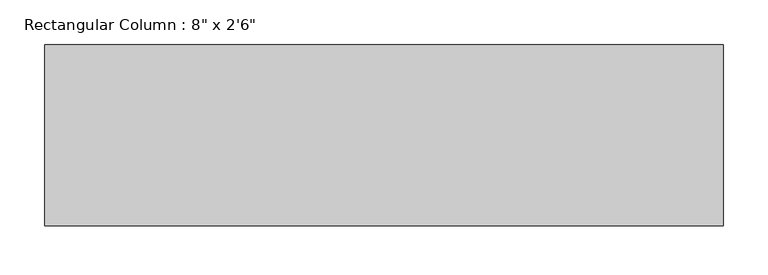
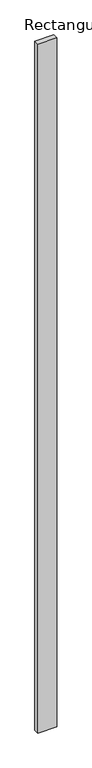
"""IFC4 building model written with IfcOpenShell, lengths in millimetres: column geometry."""

from ifc_helpers import new_model, si_unit, origin, origin_with_axes, place, context, project, spatial, polyline, outline, extrude, source, transform, mapped, element, save


def column_25705251(model_context):
    return source(origin(), model_context, "Body", "SweptSolid", [
        extrude(outline(polyline([(381.0, 101.6), (381.0, -101.6), (-381.0, -101.6), (-381.0, 101.6), (381.0, 101.6)])), origin_with_axes(), (0.0, 0.0, 1.0), 29108.4),
    ])


if __name__ == "__main__":
    model = new_model("IFC4")
    model_context = context("Model", 3, world=origin())
    ifc_project = project(units=[si_unit("LENGTHUNIT", "METRE", prefix="MILLI")], contexts=[model_context])
    site = spatial("IfcSite", under=ifc_project)
    building = spatial("IfcBuilding", under=site)
    placement = place(None, origin())
    column_shape = column_25705251(model_context)
    element("IfcColumn", 1, ObjectType="Rectangular Column : 8\" x 2'6\"", at=placement, inside=building, context=model_context, shape_type="MappedRepresentation", body=[
        mapped(column_shape, transform((0.0, 0.0, 0.0), x_axis=(1.0, 0.0, 0.0), y_axis=(0.0, 1.0, 0.0), z_axis=(0.0, 0.0, 1.0))),
    ])
    save(model, "model.ifc")

# Revit data of these elements
# Type "Rectangular Column : 8\" x 2'6\""
#   Assembly Code = "B1010200"
#   Depth = 0' - 8"
#   Offset Base = 0' - 0"
#   Offset Top = 0' - 0"
#   Width = 2' - 6"
#   Material = none
